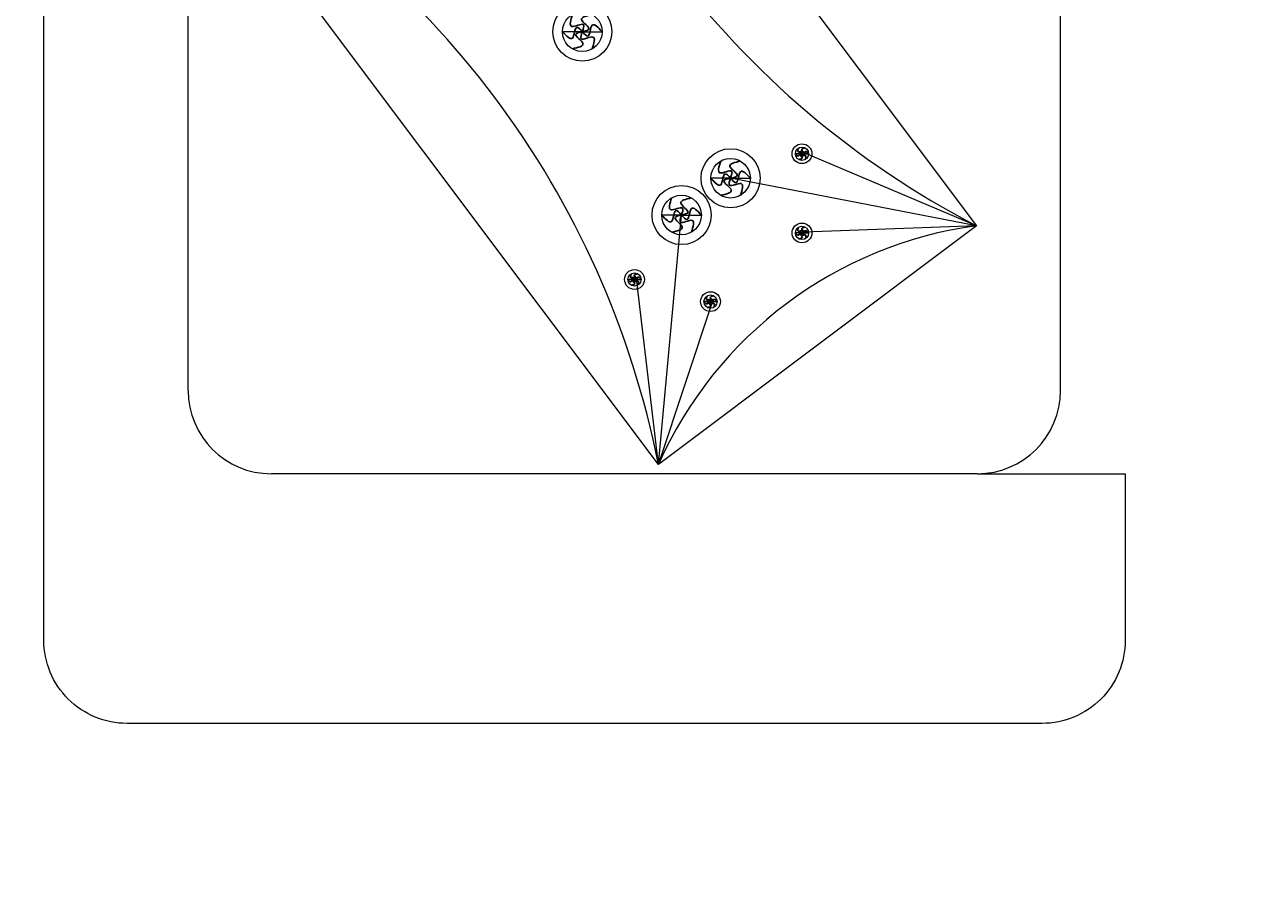
# Model space of a CAD drawing. Units: inches. Extents: x -61 to 1599, y -1316 to 257.
# Tile 128 of 204: x 388 to 418, y -143 to -122. Entities that reach past the tile are written whole.
import ezdxf

# ---------------------------------------------------------------- set-up
doc = ezdxf.new("R2010")
doc.units = ezdxf.units.IN
doc.header["$MEASUREMENT"] = 0
doc.layers.add('A-ANNO-DIMS', color=2, linetype='Continuous', lineweight=18)
doc.layers.add('FURNITURE', color=83, linetype='Continuous', lineweight=18)
doc.layers.add('FUR', color=83, linetype='Continuous')
doc.styles.get("Standard").update_dxf_attribs({"font": 'arial.ttf'})
doc.dimstyles.get("Standard").update_dxf_attribs({"dimtxt": 0.18, "dimasz": 0.18, "dimexe": 0.18, "dimexo": 0.0625, "dimgap": 0.09, "dimtad": 0, "dimtih": 1, "dimtoh": 1, "dimdec": 0, "dimzin": 0, "dimdsep": 46, "dimlunit": 3, "dimtxsty": 'Standard', "dimcen": 0.09, "dimadec": 0, "dimazin": 0, "dimtfac": 1, "dimtdec": 0, "dimtofl": 0, "dimtmove": 0, "dimatfit": 3, "dimfxl": 1, "dimtolj": 1, "dimtzin": 0, "dimarcsym": 0})

# ---------------------------------------------------------------- blocks, each defined once
blk = doc.blocks.new('*U170')
at = {"layer": 'FUR'}
blk.add_open_spline([(0.015, 0.238), (-0.088, 0.143), (-0.292, -0.045), (0.224, -0.053), (0.072, -0.187), (0.015, -0.238)], degree=3, knots=[0, 0, 0, 0, 0.2846533, 0.5662105, 0.736751, 0.736751, 0.736751, 0.736751], dxfattribs=at)
blk = doc.blocks.new('*U171')
at = {"layer": 'FUR', "transparency": 16777216}
blk.add_blockref('*U170', (662.716, -238.357), dxfattribs=at)
for p, rotation in [((662.929, -238.463), 300), ((662.517, -238.489), 60), ((662.531, -238.727), 120), ((662.944, -238.702), 240), ((662.745, -238.833), 180)]:
    blk.add_blockref('*U170', p, dxfattribs=dict(at, rotation=rotation))
blk = doc.blocks.new('*U164')
at = {"layer": 'FUR'}
blk.add_open_spline([(0.005, 0.08), (-0.03, 0.048), (-0.098, -0.015), (0.075, -0.018), (0.024, -0.063), (0.005, -0.08)], degree=3, knots=[0, 0, 0, 0, 0.0954578, 0.1898773, 0.2470677, 0.2470677, 0.2470677, 0.2470677], dxfattribs=at)
blk = doc.blocks.new('*U165')
at = {"layer": 'FUR', "transparency": 16777216}
for p, rotation in [((222.173, -79.977), 60), ((222.178, -80.056), 120), ((222.25, -80.092), 180), ((222.312, -79.968), 300), ((222.317, -80.048), 240)]:
    blk.add_blockref('*U164', p, dxfattribs=dict(at, rotation=rotation))
blk.add_blockref('*U164', (222.24, -79.932), dxfattribs=at)
blk = doc.blocks.new('*U183')
at = {"layer": 'FUR'}
blk.add_open_spline([(0.015, 0.238), (-0.088, 0.143), (-0.292, -0.045), (0.224, -0.053), (0.072, -0.187), (0.015, -0.238)], degree=3, knots=[0, 0, 0, 0, 0.2846533, 0.5662105, 0.736751, 0.736751, 0.736751, 0.736751], dxfattribs=at)
blk = doc.blocks.new('*U162')
at = {"layer": 'FUR', "transparency": 16777216}
blk.add_blockref('*U183', (662.716, -238.357), dxfattribs=at)
for p, rotation in [((662.929, -238.463), 300), ((662.517, -238.489), 60), ((662.531, -238.727), 120), ((662.944, -238.702), 240), ((662.745, -238.833), 180)]:
    blk.add_blockref('*U183', p, dxfattribs=dict(at, rotation=rotation))
blk = doc.blocks.new('*U182')
at = {"layer": 'FUR'}
blk.add_open_spline([(0.005, 0.08), (-0.03, 0.048), (-0.098, -0.015), (0.075, -0.018), (0.024, -0.063), (0.005, -0.08)], degree=3, knots=[0, 0, 0, 0, 0.0954578, 0.1898773, 0.2470677, 0.2470677, 0.2470677, 0.2470677], dxfattribs=at)
blk = doc.blocks.new('*U163')
at = {"layer": 'FUR', "transparency": 16777216}
for p, rotation in [((222.173, -79.977), 60), ((222.178, -80.056), 120), ((222.25, -80.092), 180), ((222.312, -79.968), 300), ((222.317, -80.048), 240)]:
    blk.add_blockref('*U182', p, dxfattribs=dict(at, rotation=rotation))
blk.add_blockref('*U182', (222.24, -79.932), dxfattribs=at)
blk = doc.blocks.new('*U166')
at = {"layer": 'FUR'}
blk.add_open_spline([(0.015, 0.238), (-0.088, 0.143), (-0.292, -0.045), (0.224, -0.053), (0.072, -0.187), (0.015, -0.238)], degree=3, knots=[0, 0, 0, 0, 0.2846533, 0.5662105, 0.736751, 0.736751, 0.736751, 0.736751], dxfattribs=at)
blk = doc.blocks.new('*U167')
at = {"layer": 'FUR', "transparency": 16777216}
blk.add_blockref('*U166', (662.716, -238.357), dxfattribs=at)
for p, rotation in [((662.929, -238.463), 300), ((662.517, -238.489), 60), ((662.531, -238.727), 120), ((662.944, -238.702), 240), ((662.745, -238.833), 180)]:
    blk.add_blockref('*U166', p, dxfattribs=dict(at, rotation=rotation))
blk = doc.blocks.new('*U178')
at = {"layer": 'FUR'}
blk.add_open_spline([(0.005, 0.08), (-0.03, 0.048), (-0.098, -0.015), (0.075, -0.018), (0.024, -0.063), (0.005, -0.08)], degree=3, knots=[0, 0, 0, 0, 0.0954578, 0.1898773, 0.2470677, 0.2470677, 0.2470677, 0.2470677], dxfattribs=at)
blk = doc.blocks.new('*U179')
at = {"layer": 'FUR', "transparency": 16777216}
for p, rotation in [((222.173, -79.977), 60), ((222.178, -80.056), 120), ((222.25, -80.092), 180), ((222.312, -79.968), 300), ((222.317, -80.048), 240)]:
    blk.add_blockref('*U178', p, dxfattribs=dict(at, rotation=rotation))
blk.add_blockref('*U178', (222.24, -79.932), dxfattribs=at)
blk = doc.blocks.new('*U180')
at = {"layer": 'FUR'}
blk.add_open_spline([(0.005, 0.08), (-0.03, 0.048), (-0.098, -0.015), (0.075, -0.018), (0.024, -0.063), (0.005, -0.08)], degree=3, knots=[0, 0, 0, 0, 0.0954578, 0.1898773, 0.2470677, 0.2470677, 0.2470677, 0.2470677], dxfattribs=at)
blk = doc.blocks.new('*U181')
at = {"layer": 'FUR', "transparency": 16777216}
for p, rotation in [((222.173, -79.977), 60), ((222.178, -80.056), 120), ((222.25, -80.092), 180), ((222.312, -79.968), 300), ((222.317, -80.048), 240)]:
    blk.add_blockref('*U180', p, dxfattribs=dict(at, rotation=rotation))
blk.add_blockref('*U180', (222.24, -79.932), dxfattribs=at)
blk = doc.blocks.new('SOFA-LOVESEAT')
for p, q in [((3.47, 8), (3.47, 52)), ((24.442, 8), (24.442, 28)), ((12.946, 16.624), (12.47, 16.624)), ((12.946, 16.624), (13.423, 16.624)), ((22.422, 11.961), (18.28, 13.711)), ((18.228, 13.691), (18.068, 13.691)), ((18.228, 13.691), (18.388, 13.691)), ((16.511, 13.102), (16.035, 13.102)), ((22.422, 11.961), (16.511, 13.102)), ((16.511, 13.102), (16.988, 13.102)), ((14.776, 6.223), (15.332, 12.217)), ((15.332, 12.217), (14.855, 12.217)), ((15.332, 12.217), (15.808, 12.217)), ((22.422, 11.961), (18.28, 11.807)), ((18.228, 11.787), (18.068, 11.787)), ((18.228, 11.787), (18.388, 11.787)), ((14.201, 10.669), (14.041, 10.669)), ((14.201, 10.669), (14.36, 10.669)), ((14.776, 6.223), (14.253, 10.689)), ((14.776, 6.223), (16.081, 10.156)), ((16.029, 10.137), (15.869, 10.137)), ((16.029, 10.137), (16.189, 10.137)), ((22.442, 6), (5.47, 6)), ((22.442, 6), (26, 6))]:
    blk.add_line(p, q)
blk.add_lwpolyline([(26, 6), (26, 2, -0.414214), (24, 0), (2, 0, -0.414214), (0, 2), (0, 58, -0.414213), (2, 60), (24, 60, -0.414214), (26, 58), (26, 54)], format="xyb")
blk.add_lwpolyline([(11.116, 27.026), (22.422, 11.961), (14.776, 6.223), (3.47, 21.288)], close=True)
for centre, radius in [((12.946, 16.624), 0.71), ((12.946, 16.624), 0.476), ((16.511, 13.102), 0.71), ((18.228, 13.691), 0.238), ((18.228, 13.691), 0.16), ((16.511, 13.102), 0.476), ((15.332, 12.217), 0.71), ((15.332, 12.217), 0.476), ((18.228, 11.787), 0.238), ((18.228, 11.787), 0.16), ((14.201, 10.669), 0.238), ((14.201, 10.669), 0.16), ((16.029, 10.137), 0.238), ((16.029, 10.137), 0.16)]:
    blk.add_circle(centre, radius)
for centre, radius, start, end in [((32.433, 31.248), 21.731, 191.2044, 242.5684), ((-6.541, 2), 21.731, 11.2044, 62.5684), ((23.745, 2.234), 9.816, 97.747, 156.0258), ((5.47, 8), 2, 180, 270), ((22.442, 8), 2, 270, 0)]:
    blk.add_arc(centre, radius, start, end)
at = {"rotation": 90}
for name, p in [('*U171', (-225.649, -646.106)), ('*U181', (-61.785, -208.554)), ('*U167', (-222.084, -649.628)), ('*U162', (-223.264, -650.513)), ('*U179', (-61.785, -210.458)), ('*U165', (-65.812, -211.576)), ('*U163', (-63.983, -212.108))]:
    blk.add_blockref(name, p, dxfattribs=at)
blk = doc.blocks.new('*D703')
at = {"layer": 'A-ANNO-DIMS', "color": 0, "lineweight": -2, "transparency": 16777216}
for p, q in [((372.32, -616.882), (372.32, 257.457)), ((372.5, 257.277), (413.7, 257.277)), ((455.653, 257.277), (414.453, 257.277)), ((455.833, -616.882), (455.833, 257.457))]:
    blk.add_line(p, q, dxfattribs=at)
at = {"layer": 'A-ANNO-DIMS', "color": 0, "transparency": 16777216}
for points in [[(372.5, 257.307), (372.5, 257.247), (372.32, 257.277)], [(455.653, 257.307), (455.653, 257.247), (455.833, 257.277)]]:
    blk.add_solid(points, dxfattribs=at)
at = {"layer": 'DEFPOINTS', "color": 0, "transparency": 16777216}
for p in [(455.833, 257.277), (372.32, -616.945), (455.833, -616.945)]:
    blk.add_point(p, dxfattribs=at)
at = {"layer": 'A-ANNO-DIMS', "color": 0, "transparency": 16777216, "insert": (414.076, 257.277), "char_height": 0.18, "attachment_point": 5}
blk.add_mtext('\\A1;83.51', dxfattribs=at)

msp = doc.modelspace()

# ---------------------------------------------------------------- block references
at = {"layer": 'FURNITURE'}
msp.add_blockref('SOFA-LOVESEAT', (388.9518, -138.383), dxfattribs=at)

# ---------------------------------------------------------------- dimensions: what is measured, and where the dimension line sits
at = {"layer": 'A-ANNO-DIMS'}
dim = msp.add_linear_dim(base=(455.8327, 257.2771), p1=(372.3201, -616.9446), p2=(455.8327, -616.9446), dimstyle='Standard', override={"dimdec": 2, "dimlfac": 1, "dimrnd": 0, "dimzin": 0, "dimdsep": 46, "dimlunit": 2}, dxfattribs=at)
dim.commit()
dim.dimension.update_dxf_attribs({"geometry": '*D703', "text_midpoint": (414.0764, 257.2771)})

doc.saveas('drawing.dxf')
